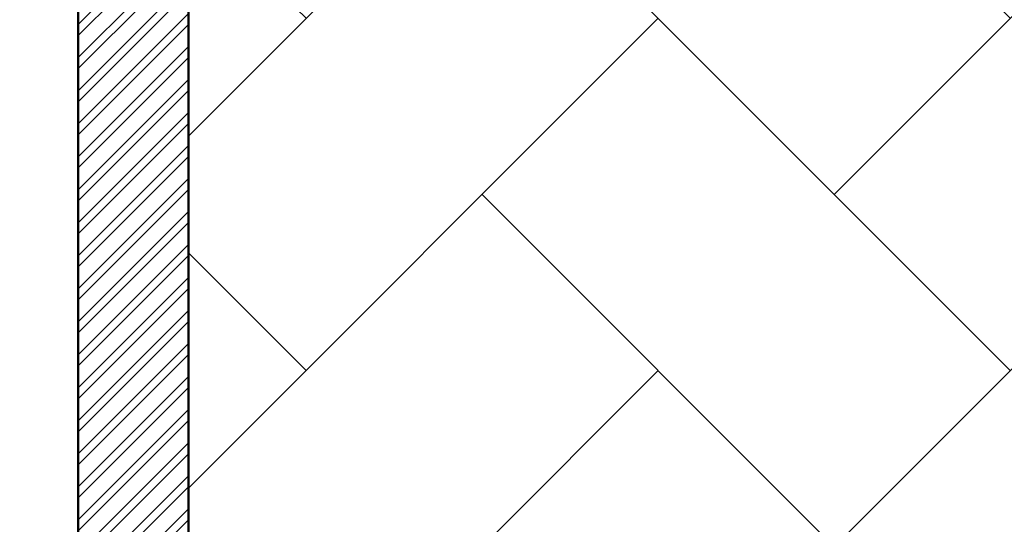
# Model space of a CAD drawing. Units: inches. Extents: x 3590 to 5167, y 65 to 1917.
# Tile 63 of 100: x 4919 to 5000, y 1640 to 1681. Entities that reach past the tile are written whole.
import ezdxf

# ---------------------------------------------------------------- set-up
doc = ezdxf.new("R2010")
doc.units = ezdxf.units.IN
for name, color, linetype, lineweight in [('A-FLOR-PATT', 8, 'Continuous', 13), ('A-WALL', 7, 'Continuous', 50), ('A-WALL-PATT', 251, 'Continuous', 13)]:
    doc.layers.add(name, color=color, linetype=linetype, lineweight=lineweight)

msp = doc.modelspace()

# ---------------------------------------------------------------- hatches: boundary and pattern name
at = {"layer": 'A-FLOR-PATT', "transparency": 33554687}
h = msp.add_hatch(dxfattribs=at)
h.set_pattern_fill('AR-HBONE', color=256, scale=0.2)
h.set_pattern_definition([(45, (-588.972, 0), (0, 28.73682), [60.96, -20.32]), (135, (-574.604, 14.368), (3e-15, 28.73682), [60.96, -20.32])])
h.paths.add_polyline_path([(5071.274, 1796.999), (4933.274, 1796.999), (4933.274, 1753.999), (4962.774, 1753.999, -0.414214), (4928.774, 1719.999), (4933.274, 1718.999), (4933.274, 1334.999), (5071.274, 1334.999)])
h.paths.add_polyline_path([(4951.78, 1521.077), (4951.715, 1521.04), (4951.563, 1520.895)], flags=16)
h.paths.add_polyline_path([(4952.267, 1521.376), (4952.198, 1521.371), (4952.198, 1521.356)], flags=0)
h.paths.add_polyline_path([(4967.051, 1529.728), (4965.231, 1528.694), (4963.411, 1527.714), (4961.756, 1526.851), (4963.589, 1527.449), (4964.036, 1527.478), (4962.975, 1527.249), (4961.76, 1526.852), (4959.792, 1525.834), (4958.005, 1524.895), (4956.24, 1523.93), (4954.504, 1522.919), (4954.129, 1522.682), (4953.361, 1521.997), (4953.366, 1521.998), (4953.605, 1522.064), (4955.106, 1522.761), (4956.921, 1523.434), (4958.678, 1523.915), (4960.358, 1524.2), (4961.945, 1524.286), (4964.171, 1524.108), (4965.958, 1523.309), (4963.863, 1522.976), (4965.187, 1522.499), (4963.366, 1522.497), (4961.545, 1522.487), (4959.764, 1522.461), (4958.304, 1522.419), (4957.974, 1522.388), (4956.307, 1522.232), (4954.718, 1522.071), (4953.251, 1521.899), (4953.525, 1521.623), (4954.331, 1521.379), (4956.243, 1521.23), (4958.039, 1520.93), (4959.684, 1520.483), (4961.16, 1519.896), (4963.107, 1518.8), (4964.393, 1517.325), (4962.973, 1517.726), (4964.558, 1516.661), (4965.407, 1515.708), (4963.507, 1516.322), (4961.68, 1517.005), (4959.935, 1517.745), (4958.282, 1518.528), (4956.732, 1519.343), (4955.295, 1520.175), (4954.672, 1520.572), (4954.513, 1520.627), (4955.658, 1519.318), (4956.703, 1517.982), (4957.644, 1516.647), (4958.485, 1515.334), (4959.55, 1513.524), (4960.438, 1511.769), (4958.841, 1513.62), (4957.452, 1515.325), (4955.819, 1517.459), (4956.665, 1515.448), (4957.111, 1513.923), (4957.447, 1511.714), (4957.076, 1509.793), (4956.538, 1511.11), (4955.992, 1512.569), (4955.444, 1514.125), (4954.898, 1515.735), (4954.357, 1517.356), (4953.824, 1518.943), (4953.305, 1520.452), (4953.065, 1521.116), (4952.971, 1521.146), (4952.949, 1521.086), (4952.73, 1520.199), (4953.37, 1518.024), (4953.757, 1516.373), (4954.051, 1514.765), (4954.264, 1513.221), (4954.471, 1511.131), (4954.497, 1510.402), (4954.409, 1511.76), (4954.264, 1513.221), (4954.051, 1514.765), (4953.757, 1516.373), (4953.37, 1518.024), (4952.877, 1519.698), (4952.716, 1520.141), (4952.533, 1519.059), (4952.374, 1517.789), (4952.219, 1516.312), (4952.046, 1514.6), (4951.833, 1512.626), (4951.557, 1510.363), (4951.203, 1512.168), (4950.852, 1514.339), (4950.985, 1516.376), (4951.66, 1518.286), (4952.593, 1520.481), (4952.357, 1521.13), (4951.855, 1520.328), (4950.839, 1518.908), (4949.777, 1517.587), (4948.916, 1516.617), (4948.111, 1515.256), (4947.089, 1513.554), (4945.889, 1511.615), (4946.326, 1513.402), (4946.562, 1514.249), (4945.528, 1513.327), (4944.581, 1512.531), (4946.018, 1514.508), (4947.204, 1516.048), (4947.893, 1517.313), (4949.307, 1518.764), (4950.414, 1519.767), (4950.451, 1519.806), (4952.267, 1521.376), (4951.645, 1521.493), (4950.404, 1521.18), (4948.044, 1520.359), (4946.119, 1519.452), (4944.572, 1518.475), (4943.35, 1517.443), (4941.997, 1515.92), (4941.661, 1515.275), (4942.813, 1516.99), (4944.572, 1518.475), (4946.119, 1519.452), (4948.044, 1520.359), (4950.404, 1521.18), (4951.645, 1521.493), (4949.647, 1521.868), (4948.6, 1521.756), (4947.126, 1521.57), (4945.42, 1521.348), (4943.45, 1521.105), (4941.183, 1520.856), (4942.86, 1521.613), (4943.873, 1522.03), (4942.952, 1521.909), (4941.41, 1521.485), (4939.543, 1520.67), (4938.968, 1520.226), (4940.733, 1521.299), (4942.952, 1521.909), (4943.702, 1522.008), (4945.894, 1522.7), (4947.565, 1522.714), (4948.921, 1522.566), (4951.131, 1522.183), (4950.971, 1522.297), (4948.129, 1523.006), (4946.035, 1523.707), (4944.232, 1524.521), (4942.707, 1525.461), (4941.444, 1526.537), (4940.43, 1527.761), (4939.649, 1529.143), (4941.421, 1528.122), (4943.147, 1527.132), (4944.841, 1526.175), (4946.514, 1525.25), (4948.179, 1524.359), (4948.365, 1524.263), (4946.475, 1526.045), (4945.181, 1527.54), (4944.19, 1529.033), (4943.496, 1530.54), (4943.278, 1531.36), (4942.498, 1531.919), (4943.114, 1531.762), (4942.959, 1533.659), (4944.14, 1531.989), (4944.612, 1531.323), (4946.202, 1530.463), (4947.486, 1529.509), (4948.79, 1528.226), (4950.368, 1526.237), (4949.485, 1528.155), (4948.851, 1530.123), (4948.491, 1532.041), (4948.381, 1533.918), (4948.501, 1535.76), (4948.827, 1537.573), (4949.418, 1535.565), (4949.957, 1533.569), (4950.464, 1531.586), (4950.961, 1529.617), (4951.391, 1527.954), (4951.724, 1530.687), (4952.201, 1532.58), (4952.889, 1534.33), (4953.77, 1535.951), (4954.827, 1537.46), (4954.521, 1535.39), (4954.273, 1533.937), (4955.58, 1535.663), (4956.748, 1536.739), (4956.159, 1534.78), (4955.589, 1532.873), (4955.043, 1531.006), (4954.525, 1529.166), (4954.038, 1527.341), (4953.638, 1525.733), (4953.611, 1525.586), (4953.398, 1524.166), (4953.382, 1524.009), (4954.07, 1525.476), (4954.912, 1527.022), (4956.136, 1528.894), (4957.847, 1530.577), (4959.376, 1531.54), (4958.256, 1530.104), (4957.143, 1528.663), (4956.066, 1527.243), (4955.056, 1525.871), (4954.141, 1524.571), (4953.352, 1523.372), (4953.311, 1523.303), (4953.273, 1522.925), (4953.261, 1522.382), (4954.103, 1523.373), (4954.63, 1524.284), (4955.961, 1526.358), (4957.23, 1528.13), (4958.421, 1529.609), (4960.037, 1531.368), (4961.374, 1532.375), (4962.101, 1532.77), (4961.07, 1531.061), (4959.987, 1529.438), (4958.869, 1527.908), (4958.15, 1527.007), (4959.803, 1528.003), (4961.589, 1528.793), (4963.391, 1529.328), (4965.211, 1529.632)], flags=16)
h.paths.add_polyline_path([(4962.944, 1523.182), (4961.107, 1523.422), (4960.392, 1523.362), (4962.35, 1523.331)], flags=0)
h.paths.add_polyline_path([(5049.541, 1584.551), (5049.476, 1584.515), (5049.325, 1584.37)], flags=16)
h.paths.add_polyline_path([(5050.028, 1584.851), (5049.959, 1584.845), (5049.959, 1584.83)], flags=0)
h.paths.add_polyline_path([(5042.333, 1581.949), (5043.88, 1582.926), (5045.806, 1583.833), (5048.165, 1584.654), (5049.406, 1584.967), (5047.408, 1585.342), (5046.361, 1585.231), (5044.888, 1585.044), (5043.181, 1584.822), (5041.211, 1584.579), (5038.944, 1584.33), (5040.622, 1585.087), (5041.634, 1585.504), (5040.713, 1585.383), (5039.171, 1584.959), (5037.304, 1584.144), (5036.729, 1583.7), (5038.494, 1584.773), (5040.713, 1585.383), (5041.463, 1585.482), (5043.655, 1586.174), (5045.326, 1586.188), (5046.682, 1586.04), (5048.893, 1585.657), (5048.732, 1585.771), (5045.891, 1586.48), (5043.796, 1587.181), (5041.994, 1587.996), (5040.468, 1588.935), (5039.205, 1590.011), (5038.191, 1591.235), (5037.41, 1592.617), (5039.182, 1591.596), (5040.909, 1590.607), (5042.602, 1589.649), (5044.275, 1588.724), (5045.94, 1587.833), (5046.126, 1587.738), (5044.237, 1589.519), (5042.942, 1591.015), (5041.952, 1592.508), (5041.257, 1594.014), (5041.039, 1594.834), (5040.26, 1595.393), (5040.875, 1595.237), (5040.721, 1597.133), (5041.901, 1595.463), (5042.373, 1594.798), (5043.963, 1593.938), (5045.247, 1592.983), (5046.552, 1591.701), (5048.129, 1589.712), (5047.247, 1591.63), (5046.613, 1593.597), (5046.252, 1595.515), (5046.142, 1597.392), (5046.262, 1599.234), (5046.588, 1601.047), (5047.179, 1599.039), (5047.718, 1597.043), (5048.225, 1595.06), (5048.722, 1593.091), (5049.152, 1591.429), (5049.485, 1594.161), (5049.962, 1596.054), (5050.65, 1597.804), (5051.532, 1599.425), (5052.589, 1600.934), (5052.283, 1598.864), (5052.034, 1597.411), (5053.341, 1599.137), (5054.509, 1600.213), (5053.92, 1598.254), (5053.35, 1596.348), (5052.805, 1594.48), (5052.286, 1592.64), (5051.799, 1590.815), (5051.4, 1589.207), (5051.373, 1589.06), (5051.159, 1587.64), (5051.143, 1587.483), (5051.831, 1588.95), (5052.673, 1590.496), (5053.898, 1592.368), (5055.608, 1594.051), (5057.137, 1595.014), (5056.017, 1593.578), (5054.904, 1592.137), (5053.828, 1590.717), (5052.817, 1589.345), (5051.902, 1588.046), (5051.113, 1586.846), (5051.072, 1586.777), (5051.034, 1586.399), (5051.022, 1585.856), (5051.864, 1586.847), (5052.391, 1587.758), (5053.723, 1589.832), (5054.991, 1591.604), (5056.182, 1593.083), (5057.798, 1594.842), (5059.135, 1595.849), (5059.863, 1596.244), (5058.831, 1594.535), (5057.749, 1592.912), (5056.63, 1591.382), (5055.912, 1590.482), (5057.564, 1591.477), (5059.35, 1592.267), (5061.152, 1592.802), (5062.972, 1593.106), (5064.812, 1593.203), (5062.992, 1592.169), (5061.172, 1591.188), (5059.518, 1590.325), (5061.35, 1590.924), (5061.797, 1590.952), (5060.737, 1590.723), (5059.521, 1590.326), (5057.553, 1589.308), (5055.766, 1588.369), (5054.002, 1587.404), (5052.265, 1586.393), (5051.891, 1586.156), (5051.122, 1585.471), (5051.127, 1585.472), (5051.366, 1585.538), (5052.867, 1586.235), (5054.682, 1586.908), (5056.439, 1587.389), (5058.12, 1587.675), (5059.706, 1587.76), (5061.933, 1587.583), (5063.719, 1586.783), (5061.624, 1586.45), (5062.949, 1585.973), (5061.127, 1585.971), (5059.307, 1585.961), (5057.525, 1585.935), (5056.065, 1585.893), (5055.735, 1585.862), (5054.068, 1585.707), (5052.479, 1585.546), (5051.012, 1585.373), (5051.286, 1585.097), (5052.092, 1584.853), (5054.004, 1584.704), (5055.8, 1584.404), (5057.446, 1583.958), (5058.921, 1583.37), (5060.868, 1582.274), (5062.154, 1580.799), (5060.734, 1581.2), (5062.32, 1580.135), (5063.168, 1579.182), (5061.269, 1579.796), (5059.441, 1580.479), (5057.696, 1581.219), (5056.043, 1582.003), (5054.493, 1582.817), (5053.057, 1583.649), (5052.433, 1584.047), (5052.274, 1584.101), (5053.42, 1582.793), (5054.464, 1581.457), (5055.405, 1580.121), (5056.247, 1578.809), (5057.311, 1576.998), (5058.199, 1575.244), (5056.602, 1577.094), (5055.213, 1578.799), (5053.58, 1580.933), (5054.427, 1578.922), (5054.872, 1577.397), (5055.208, 1575.189), (5054.838, 1573.267), (5054.299, 1574.584), (5053.754, 1576.043), (5053.206, 1577.599), (5052.659, 1579.209), (5052.118, 1580.83), (5051.585, 1582.417), (5051.066, 1583.927), (5050.826, 1584.59), (5050.733, 1584.62), (5050.711, 1584.561), (5050.491, 1583.673), (5051.131, 1581.498), (5051.518, 1579.847), (5051.813, 1578.24), (5052.026, 1576.695), (5052.233, 1574.605), (5052.258, 1573.876), (5052.17, 1575.234), (5052.026, 1576.695), (5051.813, 1578.24), (5051.518, 1579.847), (5051.131, 1581.498), (5050.638, 1583.172), (5050.477, 1583.615), (5050.294, 1582.533), (5050.136, 1581.263), (5049.981, 1579.786), (5049.807, 1578.074), (5049.594, 1576.1), (5049.318, 1573.837), (5048.965, 1575.642), (5048.613, 1577.813), (5048.747, 1579.85), (5049.421, 1581.76), (5050.354, 1583.955), (5050.118, 1584.604), (5049.616, 1583.802), (5048.6, 1582.382), (5047.538, 1581.061), (5046.677, 1580.091), (5045.872, 1578.73), (5044.85, 1577.028), (5043.651, 1575.089), (5044.087, 1576.877), (5044.324, 1577.723), (5043.289, 1576.801), (5042.342, 1576.005), (5043.779, 1577.982), (5044.966, 1579.522), (5045.655, 1580.787), (5047.068, 1582.239), (5048.175, 1583.241), (5048.213, 1583.28), (5050.028, 1584.851), (5049.406, 1584.967), (5048.165, 1584.654), (5045.806, 1583.833), (5043.88, 1582.926), (5042.333, 1581.949), (5041.111, 1580.917), (5039.758, 1579.394), (5039.423, 1578.749), (5040.575, 1580.464)], flags=16)
h.paths.add_polyline_path([(4954.799, 1533.12), (4954.262, 1532.079), (4953.831, 1530.935), (4953.505, 1529.636), (4953.283, 1528.133), (4953.167, 1526.376), (4953.156, 1524.315), (4953.277, 1521.236), (4952.802, 1521.842), (4951.557, 1521.998), (4950.976, 1521.961), (4952.661, 1521.941), (4952.802, 1521.842), (4953.152, 1523.593), (4953.167, 1526.376), (4953.283, 1528.133), (4953.609, 1530.346), (4954.456, 1532.592)], flags=0)
h.paths.add_polyline_path([(5050.563, 1585.316), (5049.318, 1585.472), (5048.737, 1585.435), (5050.422, 1585.415), (5050.563, 1585.316), (5050.914, 1587.067), (5050.928, 1589.851), (5051.045, 1591.607), (5051.371, 1593.82), (5052.217, 1596.066), (5052.56, 1596.594), (5052.024, 1595.554), (5051.592, 1594.409), (5051.266, 1593.11), (5051.045, 1591.607), (5050.928, 1589.851), (5050.918, 1587.789), (5051.038, 1584.71)], flags=0)
h.paths.add_polyline_path([(5058.153, 1586.836), (5060.111, 1586.805), (5060.705, 1586.656), (5058.868, 1586.896)], flags=0)
h.paths.add_polyline_path([(5049.541, 1430.936), (5049.476, 1430.9), (5049.325, 1430.755)], flags=16)
h.paths.add_polyline_path([(5050.028, 1431.236), (5049.959, 1431.231), (5049.959, 1431.215)], flags=0)
h.paths.add_polyline_path([(5046.588, 1447.432), (5047.179, 1445.425), (5047.718, 1443.429), (5048.225, 1441.446), (5048.722, 1439.476), (5049.152, 1437.814), (5049.485, 1440.546), (5049.962, 1442.439), (5050.65, 1444.189), (5051.532, 1445.811), (5052.589, 1447.319), (5052.283, 1445.249), (5052.034, 1443.796), (5053.341, 1445.522), (5054.509, 1446.598), (5053.92, 1444.64), (5053.35, 1442.733), (5052.805, 1440.865), (5052.286, 1439.025), (5051.799, 1437.201), (5051.4, 1435.592), (5051.373, 1435.445), (5051.159, 1434.025), (5051.143, 1433.868), (5051.831, 1435.335), (5052.673, 1436.881), (5053.898, 1438.753), (5055.608, 1440.436), (5057.137, 1441.4), (5056.017, 1439.963), (5054.904, 1438.522), (5053.828, 1437.102), (5052.817, 1435.73), (5051.902, 1434.431), (5051.113, 1433.231), (5051.072, 1433.162), (5051.034, 1432.784), (5051.022, 1432.242), (5051.864, 1433.232), (5052.391, 1434.143), (5053.723, 1436.217), (5054.991, 1437.989), (5056.182, 1439.468), (5057.798, 1441.227), (5059.135, 1442.235), (5059.863, 1442.629), (5058.831, 1440.921), (5057.749, 1439.298), (5056.63, 1437.767), (5055.912, 1436.867), (5057.564, 1437.863), (5059.35, 1438.652), (5061.152, 1439.187), (5062.972, 1439.491), (5064.812, 1439.588), (5062.992, 1438.554), (5061.172, 1437.573), (5059.518, 1436.71), (5061.35, 1437.309), (5061.797, 1437.337), (5060.737, 1437.108), (5059.521, 1436.711), (5057.553, 1435.693), (5055.766, 1434.754), (5054.002, 1433.789), (5052.265, 1432.778), (5051.891, 1432.541), (5051.122, 1431.856), (5051.127, 1431.857), (5051.366, 1431.923), (5052.867, 1432.62), (5054.682, 1433.293), (5056.439, 1433.775), (5058.12, 1434.06), (5059.706, 1434.145), (5061.933, 1433.968), (5063.719, 1433.168), (5061.624, 1432.835), (5062.949, 1432.358), (5061.127, 1432.357), (5059.307, 1432.346), (5057.525, 1432.32), (5056.065, 1432.278), (5055.735, 1432.248), (5054.068, 1432.092), (5052.479, 1431.931), (5051.012, 1431.759), (5051.286, 1431.482), (5052.092, 1431.238), (5054.004, 1431.089), (5055.8, 1430.789), (5057.446, 1430.343), (5058.921, 1429.755), (5060.868, 1428.66), (5062.154, 1427.185), (5060.734, 1427.585), (5062.32, 1426.52), (5063.168, 1425.567), (5061.269, 1426.181), (5059.441, 1426.865), (5057.696, 1427.604), (5056.043, 1428.388), (5054.493, 1429.202), (5053.057, 1430.034), (5052.433, 1430.432), (5052.274, 1430.487), (5053.42, 1429.178), (5054.464, 1427.842), (5055.405, 1426.506), (5056.247, 1425.194), (5057.311, 1423.383), (5058.199, 1421.629), (5056.602, 1423.479), (5055.213, 1425.184), (5053.58, 1427.318), (5054.427, 1425.307), (5054.872, 1423.782), (5055.208, 1421.574), (5054.838, 1419.652), (5054.299, 1420.97), (5053.754, 1422.428), (5053.206, 1423.984), (5052.659, 1425.595), (5052.118, 1427.215), (5051.585, 1428.802), (5051.066, 1430.312), (5050.826, 1430.975), (5050.733, 1431.005), (5050.711, 1430.946), (5050.491, 1430.058), (5051.131, 1427.883), (5051.518, 1426.232), (5051.813, 1424.625), (5052.026, 1423.081), (5052.233, 1420.991), (5052.258, 1420.261), (5052.17, 1421.619), (5052.026, 1423.081), (5051.813, 1424.625), (5051.518, 1426.232), (5051.131, 1427.883), (5050.638, 1429.558), (5050.477, 1430.001), (5050.294, 1428.918), (5050.136, 1427.648), (5049.981, 1426.171), (5049.807, 1424.459), (5049.594, 1422.485), (5049.318, 1420.222), (5048.965, 1422.028), (5048.613, 1424.199), (5048.747, 1426.235), (5049.421, 1428.146), (5050.354, 1430.34), (5050.118, 1430.989), (5049.616, 1430.187), (5048.6, 1428.768), (5047.538, 1427.446), (5046.677, 1426.477), (5045.872, 1425.116), (5044.85, 1423.413), (5043.651, 1421.474), (5044.087, 1423.262), (5044.324, 1424.109), (5043.289, 1423.186), (5042.342, 1422.391), (5043.779, 1424.368), (5044.966, 1425.907), (5045.655, 1427.173), (5047.068, 1428.624), (5048.175, 1429.627), (5048.213, 1429.666), (5050.028, 1431.236), (5049.406, 1431.353), (5048.165, 1431.039), (5045.806, 1430.218), (5043.88, 1429.311), (5042.333, 1428.334), (5041.111, 1427.302), (5039.758, 1425.779), (5039.423, 1425.134), (5040.575, 1426.849), (5042.333, 1428.334), (5043.88, 1429.311), (5045.806, 1430.218), (5048.165, 1431.039), (5049.406, 1431.353), (5047.408, 1431.727), (5046.361, 1431.616), (5044.888, 1431.429), (5043.181, 1431.207), (5041.211, 1430.964), (5038.944, 1430.715), (5040.622, 1431.472), (5041.634, 1431.89), (5040.713, 1431.769), (5039.171, 1431.345), (5037.304, 1430.53), (5036.729, 1430.085), (5038.494, 1431.158), (5040.713, 1431.769), (5041.463, 1431.867), (5043.655, 1432.559), (5045.326, 1432.573), (5046.682, 1432.425), (5048.893, 1432.042), (5048.732, 1432.156), (5045.891, 1432.865), (5043.796, 1433.566), (5041.994, 1434.381), (5040.468, 1435.321), (5039.205, 1436.396), (5038.191, 1437.62), (5037.41, 1439.002), (5039.182, 1437.982), (5040.909, 1436.992), (5042.602, 1436.034), (5044.275, 1435.109), (5045.94, 1434.218), (5046.126, 1434.123), (5044.237, 1435.904), (5042.942, 1437.4), (5041.952, 1438.893), (5041.257, 1440.399), (5041.039, 1441.219), (5040.26, 1441.778), (5040.875, 1441.622), (5040.721, 1443.518), (5041.901, 1441.848), (5042.373, 1441.183), (5043.963, 1440.323), (5045.247, 1439.369), (5046.552, 1438.086), (5048.129, 1436.097), (5047.247, 1438.015), (5046.613, 1439.982), (5046.252, 1441.901), (5046.142, 1443.778), (5046.262, 1445.619)], flags=16)
h.paths.add_polyline_path([(5052.382, 1444.255), (5051.623, 1442.78), (5052.024, 1441.939), (5052.56, 1442.98)], flags=0)
h.paths.add_polyline_path([(5050.563, 1431.701), (5049.318, 1431.857), (5048.737, 1431.821), (5050.422, 1431.8)], flags=0)
h.paths.add_polyline_path([(5058.153, 1433.221), (5060.111, 1433.19), (5060.705, 1433.041), (5058.868, 1433.281)], flags=0)
h.paths.add_polyline_path([(5049.541, 1352.285), (5049.476, 1352.249), (5049.325, 1352.104)], flags=16)
h.paths.add_polyline_path([(5050.028, 1352.585), (5049.959, 1352.58), (5049.959, 1352.564)], flags=0)
h.paths.add_polyline_path([(5046.588, 1368.781), (5047.179, 1366.774), (5047.718, 1364.778), (5048.225, 1362.795), (5048.722, 1360.825), (5049.152, 1359.163), (5049.485, 1361.896), (5049.962, 1363.789), (5050.65, 1365.538), (5051.532, 1367.16), (5052.589, 1368.669), (5052.283, 1366.598), (5052.034, 1365.145), (5053.341, 1366.871), (5054.509, 1367.947), (5053.92, 1365.989), (5053.35, 1364.082), (5052.805, 1362.214), (5052.286, 1360.374), (5051.799, 1358.55), (5051.4, 1356.942), (5051.373, 1356.794), (5051.159, 1355.374), (5051.143, 1355.218), (5051.831, 1356.684), (5052.673, 1358.23), (5053.898, 1360.102), (5055.608, 1361.786), (5057.137, 1362.749), (5056.017, 1361.313), (5054.904, 1359.872), (5053.828, 1358.452), (5052.817, 1357.079), (5051.902, 1355.78), (5051.113, 1354.581), (5051.072, 1354.512), (5051.034, 1354.133), (5051.022, 1353.591), (5051.864, 1354.581), (5052.391, 1355.492), (5053.723, 1357.566), (5054.991, 1359.338), (5056.182, 1360.817), (5057.798, 1362.577), (5059.135, 1363.584), (5059.863, 1363.979), (5058.831, 1362.27), (5057.749, 1360.647), (5056.63, 1359.117), (5055.912, 1358.216), (5057.564, 1359.212), (5059.35, 1360.001), (5061.152, 1360.536), (5062.972, 1360.841), (5064.812, 1360.937), (5062.992, 1359.903), (5061.172, 1358.923), (5059.518, 1358.059), (5061.35, 1358.658), (5061.797, 1358.687), (5060.737, 1358.458), (5059.521, 1358.061), (5057.553, 1357.043), (5055.766, 1356.103), (5054.002, 1355.138), (5052.265, 1354.127), (5051.891, 1353.89), (5051.122, 1353.206), (5051.127, 1353.206), (5051.366, 1353.272), (5052.867, 1353.969), (5054.682, 1354.643), (5056.439, 1355.124), (5058.12, 1355.409), (5059.706, 1355.495), (5061.933, 1355.317), (5063.719, 1354.518), (5061.624, 1354.184), (5062.949, 1353.708), (5061.127, 1353.706), (5059.307, 1353.695), (5057.525, 1353.669), (5056.065, 1353.627), (5055.735, 1353.597), (5054.068, 1353.441), (5052.479, 1353.28), (5051.012, 1353.108), (5051.286, 1352.831), (5052.092, 1352.587), (5054.004, 1352.439), (5055.8, 1352.138), (5057.446, 1351.692), (5058.921, 1351.104), (5060.868, 1350.009), (5062.154, 1348.534), (5060.734, 1348.935), (5062.32, 1347.869), (5063.168, 1346.916), (5061.269, 1347.53), (5059.441, 1348.214), (5057.696, 1348.954), (5056.043, 1349.737), (5054.493, 1350.551), (5053.057, 1351.383), (5052.433, 1351.781), (5052.274, 1351.836), (5053.42, 1350.527), (5054.464, 1349.191), (5055.405, 1347.855), (5056.247, 1346.543), (5057.311, 1344.733), (5058.199, 1342.978), (5056.602, 1344.828), (5055.213, 1346.534), (5053.58, 1348.667), (5054.427, 1346.656), (5054.872, 1345.132), (5055.208, 1342.923), (5054.838, 1341.002), (5054.299, 1342.319), (5053.754, 1343.778), (5053.206, 1345.334), (5052.659, 1346.944), (5052.118, 1348.564), (5051.585, 1350.151), (5051.066, 1351.661), (5050.826, 1352.324), (5050.733, 1352.355), (5050.711, 1352.295), (5050.491, 1351.408), (5051.131, 1349.232), (5051.518, 1347.581), (5051.813, 1345.974), (5052.026, 1344.43), (5052.233, 1342.34), (5052.258, 1341.61), (5052.17, 1342.969), (5052.026, 1344.43), (5051.813, 1345.974), (5051.518, 1347.581), (5051.131, 1349.232), (5050.638, 1350.907), (5050.477, 1351.35), (5050.294, 1350.267), (5050.136, 1348.997), (5049.981, 1347.52), (5049.807, 1345.809), (5049.594, 1343.835), (5049.318, 1341.571), (5048.965, 1343.377), (5048.613, 1345.548), (5048.747, 1347.585), (5049.421, 1349.495), (5050.354, 1351.689), (5050.118, 1352.339), (5049.616, 1351.536), (5048.6, 1350.117), (5047.538, 1348.795), (5046.677, 1347.826), (5045.872, 1346.465), (5044.85, 1344.763), (5043.651, 1342.824), (5044.087, 1344.611), (5044.324, 1345.458), (5043.289, 1344.535), (5042.342, 1343.74), (5043.779, 1345.717), (5044.966, 1347.256), (5045.655, 1348.522), (5047.068, 1349.973), (5048.175, 1350.976), (5048.213, 1351.015), (5050.028, 1352.585), (5049.406, 1352.702), (5048.165, 1352.388), (5045.806, 1351.567), (5043.88, 1350.661), (5042.333, 1349.683), (5041.111, 1348.651), (5039.758, 1347.128), (5039.423, 1346.483), (5040.575, 1348.198), (5042.333, 1349.683), (5043.88, 1350.661), (5045.806, 1351.567), (5048.165, 1352.388), (5049.406, 1352.702), (5047.408, 1353.076), (5046.361, 1352.965), (5044.888, 1352.779), (5043.181, 1352.556), (5041.211, 1352.313), (5038.944, 1352.065), (5040.622, 1352.821), (5041.634, 1353.239), (5040.713, 1353.118), (5039.171, 1352.694), (5037.304, 1351.879), (5036.729, 1351.434), (5038.494, 1352.508), (5040.713, 1353.118), (5041.463, 1353.216), (5043.655, 1353.909), (5045.326, 1353.923), (5046.682, 1353.774), (5048.893, 1353.391), (5048.732, 1353.506), (5045.891, 1354.214), (5043.796, 1354.915), (5041.994, 1355.73), (5040.468, 1356.67), (5039.205, 1357.746), (5038.191, 1358.969), (5037.41, 1360.352), (5039.182, 1359.331), (5040.909, 1358.341), (5042.602, 1357.383), (5044.275, 1356.458), (5045.94, 1355.567), (5046.126, 1355.472), (5044.237, 1357.253), (5042.942, 1358.749), (5041.952, 1360.242), (5041.257, 1361.748), (5041.039, 1362.568), (5040.26, 1363.128), (5040.875, 1362.971), (5040.721, 1364.867), (5041.901, 1363.197), (5042.373, 1362.532), (5043.963, 1361.672), (5045.247, 1360.718), (5046.552, 1359.435), (5048.129, 1357.446), (5047.247, 1359.364), (5046.613, 1361.331), (5046.252, 1363.25), (5046.142, 1365.127), (5046.262, 1366.969)], flags=16)
h.paths.add_polyline_path([(5052.382, 1365.604), (5051.623, 1364.129), (5052.024, 1363.288), (5052.56, 1364.329)], flags=0)
h.paths.add_polyline_path([(4951.78, 1698.041), (4951.715, 1698.005), (4951.563, 1697.859)], flags=16)
h.paths.add_polyline_path([(4952.267, 1698.341), (4952.198, 1698.335), (4952.198, 1698.32)], flags=0)
h.paths.add_polyline_path([(4957.076, 1686.757), (4956.538, 1688.074), (4955.992, 1689.533), (4955.444, 1691.089), (4954.898, 1692.699), (4954.357, 1694.32), (4953.824, 1695.907), (4953.305, 1697.417), (4953.065, 1698.08), (4952.971, 1698.11), (4952.949, 1698.051), (4952.73, 1697.163), (4953.37, 1694.988), (4953.757, 1693.337), (4954.051, 1691.729), (4954.264, 1690.185), (4954.471, 1688.095), (4954.497, 1687.366), (4954.409, 1688.724), (4954.264, 1690.185), (4954.051, 1691.729), (4953.757, 1693.337), (4953.37, 1694.988), (4952.877, 1696.662), (4952.716, 1697.105), (4952.533, 1696.023), (4952.374, 1694.753), (4952.219, 1693.276), (4952.046, 1691.564), (4951.833, 1689.59), (4951.557, 1687.327), (4951.203, 1689.132), (4950.852, 1691.303), (4950.985, 1693.34), (4951.66, 1695.25), (4952.593, 1697.445), (4952.357, 1698.094), (4951.855, 1697.292), (4950.839, 1695.872), (4949.777, 1694.551), (4948.916, 1693.581), (4948.111, 1692.22), (4947.089, 1690.518), (4945.889, 1688.579), (4946.326, 1690.366), (4946.562, 1691.213), (4945.528, 1690.291), (4944.581, 1689.495), (4946.018, 1691.472), (4947.204, 1693.012), (4947.893, 1694.277), (4949.307, 1695.729), (4950.414, 1696.731), (4950.451, 1696.77), (4952.267, 1698.341), (4951.645, 1698.457), (4950.404, 1698.144), (4948.044, 1697.323), (4946.119, 1696.416), (4944.572, 1695.439), (4943.35, 1694.407), (4941.997, 1692.884), (4941.661, 1692.239), (4942.813, 1693.954), (4944.572, 1695.439), (4946.119, 1696.416), (4948.044, 1697.323), (4950.404, 1698.144), (4951.645, 1698.457), (4949.647, 1698.832), (4948.6, 1698.72), (4947.126, 1698.534), (4945.42, 1698.312), (4943.45, 1698.069), (4941.183, 1697.82), (4942.86, 1698.577), (4943.873, 1698.994), (4942.952, 1698.873), (4941.41, 1698.449), (4939.543, 1697.634), (4938.968, 1697.19), (4940.733, 1698.263), (4942.952, 1698.873), (4943.702, 1698.972), (4945.894, 1699.664), (4947.565, 1699.678), (4948.921, 1699.53), (4951.131, 1699.147), (4950.971, 1699.261), (4948.129, 1699.97), (4946.035, 1700.671), (4944.232, 1701.486), (4942.707, 1702.425), (4941.444, 1703.501), (4940.43, 1704.725), (4939.649, 1706.107), (4941.421, 1705.086), (4943.147, 1704.097), (4944.841, 1703.139), (4946.514, 1702.214), (4948.179, 1701.323), (4948.365, 1701.227), (4946.475, 1703.009), (4945.181, 1704.505), (4944.19, 1705.997), (4943.496, 1707.504), (4943.278, 1708.324), (4942.498, 1708.883), (4943.114, 1708.727), (4942.959, 1710.623), (4944.14, 1708.953), (4944.612, 1708.287), (4946.202, 1707.428), (4947.486, 1706.473), (4948.79, 1705.191), (4950.368, 1703.202), (4949.485, 1705.12), (4948.851, 1707.087), (4948.491, 1709.005), (4948.381, 1710.882), (4948.501, 1712.724), (4948.827, 1714.537), (4949.418, 1712.529), (4949.957, 1710.533), (4950.464, 1708.55), (4950.961, 1706.581), (4951.391, 1704.919), (4951.724, 1707.651), (4952.201, 1709.544), (4952.889, 1711.294), (4953.77, 1712.915), (4954.827, 1714.424), (4954.521, 1712.354), (4954.273, 1710.901), (4955.58, 1712.627), (4956.748, 1713.703), (4956.159, 1711.744), (4955.589, 1709.837), (4955.043, 1707.97), (4954.525, 1706.13), (4954.038, 1704.305), (4953.638, 1702.697), (4953.611, 1702.55), (4953.398, 1701.13), (4953.382, 1700.973), (4954.07, 1702.44), (4954.912, 1703.986), (4956.136, 1705.858), (4957.847, 1707.541), (4959.376, 1708.504), (4958.256, 1707.068), (4957.143, 1705.627), (4956.066, 1704.207), (4955.056, 1702.835), (4954.141, 1701.536), (4953.352, 1700.336), (4953.311, 1700.267), (4953.273, 1699.889), (4953.261, 1699.346), (4954.103, 1700.337), (4954.63, 1701.248), (4955.961, 1703.322), (4957.23, 1705.094), (4958.421, 1706.573), (4960.037, 1708.332), (4961.374, 1709.339), (4962.101, 1709.734), (4961.07, 1708.025), (4959.987, 1706.402), (4958.869, 1704.872), (4958.15, 1703.972), (4959.803, 1704.967), (4961.589, 1705.757), (4963.391, 1706.292), (4965.211, 1706.596), (4967.051, 1706.692), (4965.231, 1705.659), (4963.411, 1704.678), (4961.756, 1703.815), (4963.589, 1704.413), (4964.036, 1704.442), (4962.975, 1704.213), (4961.76, 1703.816), (4959.792, 1702.798), (4958.005, 1701.859), (4956.24, 1700.894), (4954.504, 1699.883), (4954.129, 1699.646), (4953.361, 1698.961), (4953.366, 1698.962), (4953.605, 1699.028), (4955.106, 1699.725), (4956.921, 1700.398), (4958.678, 1700.879), (4960.358, 1701.164), (4961.945, 1701.25), (4964.171, 1701.073), (4965.958, 1700.273), (4963.863, 1699.94), (4965.187, 1699.463), (4963.366, 1699.461), (4961.545, 1699.451), (4959.764, 1699.425), (4958.304, 1699.383), (4957.974, 1699.352), (4956.307, 1699.197), (4954.718, 1699.036), (4953.251, 1698.863), (4953.525, 1698.587), (4954.331, 1698.343), (4956.243, 1698.194), (4958.039, 1697.894), (4959.684, 1697.447), (4961.16, 1696.86), (4963.107, 1695.764), (4964.393, 1694.289), (4962.973, 1694.69), (4964.558, 1693.625), (4965.407, 1692.672), (4963.507, 1693.286), (4961.68, 1693.969), (4959.935, 1694.709), (4958.282, 1695.492), (4956.732, 1696.307), (4955.295, 1697.139), (4954.672, 1697.536), (4954.513, 1697.591), (4955.658, 1696.282), (4956.703, 1694.946), (4957.644, 1693.611), (4958.485, 1692.298), (4959.55, 1690.488), (4960.438, 1688.733), (4958.841, 1690.584), (4957.452, 1692.289), (4955.819, 1694.423), (4956.665, 1692.412), (4957.111, 1690.887), (4957.447, 1688.678)], flags=16)
h.paths.add_polyline_path([(5050.563, 1353.05), (5049.318, 1353.207), (5048.737, 1353.17), (5050.422, 1353.15)], flags=0)
h.paths.add_polyline_path([(4951.78, 1351.486), (4951.715, 1351.45), (4951.563, 1351.305)], flags=16)
h.paths.add_polyline_path([(4952.267, 1351.786), (4952.198, 1351.78), (4952.198, 1351.765)], flags=0)
h.paths.add_polyline_path([(4954.827, 1367.869), (4954.521, 1365.799), (4954.273, 1364.346), (4955.58, 1366.072), (4956.748, 1367.148), (4956.159, 1365.19), (4955.589, 1363.283), (4955.043, 1361.415), (4954.525, 1359.575), (4954.038, 1357.751), (4953.638, 1356.142), (4953.611, 1355.995), (4953.398, 1354.575), (4953.382, 1354.418), (4954.07, 1355.885), (4954.912, 1357.431), (4956.136, 1359.303), (4957.847, 1360.986), (4959.376, 1361.95), (4958.256, 1360.513), (4957.143, 1359.072), (4956.066, 1357.652), (4955.056, 1356.28), (4954.141, 1354.981), (4953.352, 1353.781), (4953.311, 1353.712), (4953.273, 1353.334), (4953.261, 1352.792), (4954.103, 1353.782), (4954.63, 1354.693), (4955.961, 1356.767), (4957.23, 1358.539), (4958.421, 1360.018), (4960.037, 1361.777), (4961.374, 1362.785), (4962.101, 1363.179), (4961.07, 1361.471), (4959.987, 1359.848), (4958.869, 1358.317), (4958.15, 1357.417), (4959.803, 1358.413), (4961.589, 1359.202), (4963.391, 1359.737), (4965.211, 1360.041), (4967.051, 1360.138), (4965.231, 1359.104), (4963.411, 1358.123), (4961.756, 1357.26), (4963.589, 1357.859), (4964.036, 1357.887), (4962.975, 1357.658), (4961.76, 1357.261), (4959.792, 1356.243), (4958.005, 1355.304), (4956.24, 1354.339), (4954.504, 1353.328), (4954.129, 1353.091), (4953.361, 1352.406), (4953.366, 1352.407), (4953.605, 1352.473), (4955.106, 1353.17), (4956.921, 1353.843), (4958.678, 1354.325), (4960.358, 1354.61), (4961.945, 1354.695), (4964.171, 1354.518), (4965.958, 1353.718), (4963.863, 1353.385), (4965.187, 1352.908), (4963.366, 1352.907), (4961.545, 1352.896), (4959.764, 1352.87), (4958.304, 1352.828), (4957.974, 1352.798), (4956.307, 1352.642), (4954.718, 1352.481), (4953.251, 1352.309), (4953.525, 1352.032), (4954.331, 1351.788), (4956.243, 1351.639), (4958.039, 1351.339), (4959.684, 1350.893), (4961.16, 1350.305), (4963.107, 1349.21), (4964.393, 1347.735), (4962.973, 1348.135), (4964.558, 1347.07), (4965.407, 1346.117), (4963.507, 1346.731), (4961.68, 1347.414), (4959.935, 1348.154), (4958.282, 1348.938), (4956.732, 1349.752), (4955.295, 1350.584), (4954.672, 1350.982), (4954.513, 1351.036), (4955.658, 1349.728), (4956.703, 1348.392), (4957.644, 1347.056), (4958.485, 1345.744), (4959.55, 1343.933), (4960.438, 1342.179), (4958.841, 1344.029), (4957.452, 1345.734), (4955.819, 1347.868), (4956.665, 1345.857), (4957.111, 1344.332), (4957.447, 1342.124), (4957.076, 1340.202), (4956.538, 1341.52), (4955.992, 1342.978), (4955.444, 1344.534), (4954.898, 1346.145), (4954.357, 1347.765), (4953.824, 1349.352), (4953.305, 1350.862), (4953.065, 1351.525), (4952.971, 1351.555), (4952.949, 1351.496), (4952.73, 1350.608), (4953.37, 1348.433), (4953.757, 1346.782), (4954.051, 1345.175), (4954.264, 1343.631), (4954.471, 1341.541), (4954.497, 1340.811), (4954.409, 1342.169), (4954.264, 1343.631), (4954.051, 1345.175), (4953.757, 1346.782), (4953.37, 1348.433), (4952.877, 1350.108), (4952.716, 1350.551), (4952.533, 1349.468), (4952.374, 1348.198), (4952.219, 1346.721), (4952.046, 1345.009), (4951.833, 1343.035), (4951.557, 1340.772), (4951.203, 1342.578), (4950.852, 1344.749), (4950.985, 1346.785), (4951.66, 1348.696), (4952.593, 1350.89), (4952.357, 1351.539), (4951.855, 1350.737), (4950.839, 1349.318), (4949.777, 1347.996), (4948.916, 1347.027), (4948.111, 1345.665), (4947.089, 1343.963), (4945.889, 1342.024), (4946.326, 1343.812), (4946.562, 1344.659), (4945.528, 1343.736), (4944.581, 1342.941), (4946.018, 1344.918), (4947.204, 1346.457), (4947.893, 1347.723), (4949.307, 1349.174), (4950.414, 1350.177), (4950.451, 1350.216), (4952.267, 1351.786), (4951.645, 1351.903), (4950.404, 1351.589), (4948.044, 1350.768), (4946.119, 1349.861), (4944.572, 1348.884), (4943.35, 1347.852), (4941.997, 1346.329), (4941.661, 1345.684), (4942.813, 1347.399), (4944.572, 1348.884), (4946.119, 1349.861), (4948.044, 1350.768), (4950.404, 1351.589), (4951.645, 1351.903), (4949.647, 1352.277), (4948.6, 1352.166), (4947.126, 1351.979), (4945.42, 1351.757), (4943.45, 1351.514), (4941.183, 1351.265), (4942.86, 1352.022), (4943.873, 1352.44), (4942.952, 1352.319), (4941.41, 1351.895), (4939.543, 1351.08), (4938.968, 1350.635), (4940.733, 1351.708), (4942.952, 1352.319), (4943.702, 1352.417), (4945.894, 1353.109), (4947.565, 1353.123), (4948.921, 1352.975), (4951.131, 1352.592), (4950.971, 1352.706), (4948.129, 1353.415), (4946.035, 1354.116), (4944.232, 1354.931), (4942.707, 1355.871), (4941.444, 1356.946), (4940.43, 1358.17), (4939.649, 1359.552), (4941.421, 1358.532), (4943.147, 1357.542), (4944.841, 1356.584), (4946.514, 1355.659), (4948.179, 1354.768), (4948.365, 1354.673), (4946.475, 1356.454), (4945.181, 1357.95), (4944.19, 1359.443), (4943.496, 1360.949), (4943.278, 1361.769), (4942.498, 1362.328), (4943.114, 1362.172), (4942.959, 1364.068), (4944.14, 1362.398), (4944.612, 1361.733), (4946.202, 1360.873), (4947.486, 1359.919), (4948.79, 1358.636), (4950.368, 1356.647), (4949.485, 1358.565), (4948.851, 1360.532), (4948.491, 1362.451), (4948.381, 1364.328), (4948.501, 1366.169), (4948.827, 1367.982), (4949.418, 1365.975), (4949.957, 1363.979), (4950.464, 1361.995), (4950.961, 1360.026), (4951.391, 1358.364), (4951.724, 1361.096), (4952.201, 1362.989), (4952.889, 1364.739), (4953.77, 1366.361)], flags=16)
h.paths.add_polyline_path([(4954.799, 1363.53), (4954.262, 1362.489), (4953.831, 1361.344), (4953.505, 1360.045), (4953.283, 1358.543), (4953.167, 1356.786), (4953.156, 1354.724), (4953.277, 1351.646), (4952.802, 1352.251), (4951.557, 1352.407), (4950.976, 1352.371), (4952.661, 1352.35), (4952.802, 1352.251), (4953.152, 1354.002), (4953.167, 1356.786), (4953.283, 1358.543), (4953.609, 1360.755), (4954.456, 1363.001)], flags=0)
h.paths.add_polyline_path([(4952.802, 1698.806), (4951.557, 1698.962), (4950.976, 1698.925), (4952.661, 1698.905), (4952.802, 1698.806), (4953.152, 1700.557), (4953.167, 1703.34), (4953.283, 1705.097), (4953.609, 1707.31), (4954.456, 1709.556), (4954.799, 1710.084), (4954.262, 1709.043), (4953.831, 1707.899), (4953.505, 1706.6), (4953.283, 1705.097), (4953.167, 1703.34), (4953.156, 1701.279), (4953.277, 1698.2)], flags=0)
h.paths.add_polyline_path([(4962.944, 1700.146), (4961.107, 1700.386), (4960.392, 1700.326), (4962.35, 1700.295)], flags=0)
h.paths.add_polyline_path([(5058.153, 1354.57), (5060.111, 1354.539), (5060.705, 1354.391), (5058.868, 1354.631)], flags=0)
h.paths.add_polyline_path([(4962.944, 1353.591), (4961.107, 1353.831), (4960.392, 1353.771), (4962.35, 1353.74)], flags=0)
h.paths.add_polyline_path([(5049.541, 1778.72), (5049.476, 1778.684), (5049.325, 1778.539)], flags=16)
h.paths.add_polyline_path([(5050.028, 1779.02), (5049.959, 1779.014), (5049.959, 1778.999)], flags=0)
h.paths.add_polyline_path([(5052.258, 1768.045), (5052.17, 1769.403), (5052.026, 1770.864), (5051.813, 1772.409), (5051.518, 1774.016), (5051.131, 1775.667), (5050.638, 1777.341), (5050.477, 1777.784), (5050.294, 1776.702), (5050.136, 1775.432), (5049.981, 1773.955), (5049.807, 1772.243), (5049.594, 1770.269), (5049.318, 1768.006), (5048.965, 1769.811), (5048.613, 1771.982), (5048.747, 1774.019), (5049.421, 1775.929), (5050.354, 1778.124), (5050.118, 1778.773), (5049.616, 1777.971), (5048.6, 1776.551), (5047.538, 1775.23), (5046.677, 1774.26), (5045.872, 1772.899), (5044.85, 1771.197), (5043.651, 1769.258), (5044.087, 1771.046), (5044.324, 1771.892), (5043.289, 1770.97), (5042.342, 1770.174), (5043.779, 1772.151), (5044.966, 1773.691), (5045.655, 1774.956), (5047.068, 1776.408), (5048.175, 1777.41), (5048.213, 1777.449), (5050.028, 1779.02), (5049.406, 1779.136), (5048.165, 1778.823), (5045.806, 1778.002), (5043.88, 1777.095), (5042.333, 1776.118), (5041.111, 1775.086), (5039.758, 1773.563), (5039.423, 1772.918), (5040.575, 1774.633), (5042.333, 1776.118), (5043.88, 1777.095), (5045.806, 1778.002), (5048.165, 1778.823), (5049.406, 1779.136), (5047.408, 1779.511), (5046.361, 1779.4), (5044.888, 1779.213), (5043.181, 1778.991), (5041.211, 1778.748), (5038.944, 1778.499), (5040.622, 1779.256), (5041.634, 1779.673), (5040.713, 1779.552), (5039.171, 1779.128), (5037.304, 1778.313), (5036.729, 1777.869), (5038.494, 1778.942), (5040.713, 1779.552), (5041.463, 1779.651), (5043.655, 1780.343), (5045.326, 1780.357), (5046.682, 1780.209), (5048.893, 1779.826), (5048.732, 1779.94), (5045.891, 1780.649), (5043.796, 1781.35), (5041.994, 1782.165), (5040.468, 1783.104), (5039.205, 1784.18), (5038.191, 1785.404), (5037.41, 1786.786), (5039.182, 1785.765), (5040.909, 1784.776), (5042.602, 1783.818), (5044.275, 1782.893), (5045.94, 1782.002), (5046.126, 1781.907), (5044.237, 1783.688), (5042.942, 1785.184), (5041.952, 1786.677), (5041.257, 1788.183), (5041.039, 1789.003), (5040.26, 1789.562), (5040.875, 1789.406), (5040.721, 1791.302), (5041.901, 1789.632), (5042.373, 1788.967), (5043.963, 1788.107), (5045.247, 1787.152), (5046.552, 1785.87), (5048.129, 1783.881), (5047.247, 1785.799), (5046.613, 1787.766), (5046.252, 1789.684), (5046.142, 1791.561), (5046.262, 1793.403), (5046.588, 1795.216), (5047.179, 1793.208), (5047.718, 1791.213), (5048.225, 1789.229), (5048.722, 1787.26), (5049.152, 1785.598), (5049.485, 1788.33), (5049.962, 1790.223), (5050.65, 1791.973), (5051.532, 1793.594), (5052.589, 1795.103), (5052.283, 1793.033), (5052.034, 1791.58), (5053.341, 1793.306), (5054.509, 1794.382), (5053.92, 1792.423), (5053.35, 1790.517), (5052.805, 1788.649), (5052.286, 1786.809), (5051.799, 1784.984), (5051.4, 1783.376), (5051.373, 1783.229), (5051.159, 1781.809), (5051.143, 1781.652), (5051.831, 1783.119), (5052.673, 1784.665), (5053.898, 1786.537), (5055.608, 1788.22), (5057.137, 1789.183), (5056.017, 1787.747), (5054.904, 1786.306), (5053.828, 1784.886), (5052.817, 1783.514), (5051.902, 1782.215), (5051.113, 1781.015), (5051.072, 1780.946), (5051.034, 1780.568), (5051.022, 1780.025), (5051.864, 1781.016), (5052.391, 1781.927), (5053.723, 1784.001), (5054.991, 1785.773), (5056.182, 1787.252), (5057.798, 1789.011), (5059.135, 1790.018), (5059.863, 1790.413), (5058.831, 1788.704), (5057.749, 1787.081), (5056.63, 1785.551), (5055.912, 1784.651), (5057.564, 1785.646), (5059.35, 1786.436), (5061.152, 1786.971), (5062.972, 1787.275), (5064.812, 1787.372), (5062.992, 1786.338), (5061.172, 1785.357), (5059.518, 1784.494), (5061.35, 1785.093), (5061.797, 1785.121), (5060.737, 1784.892), (5059.521, 1784.495), (5057.553, 1783.477), (5055.766, 1782.538), (5054.002, 1781.573), (5052.265, 1780.562), (5051.891, 1780.325), (5051.122, 1779.64), (5051.127, 1779.641), (5051.366, 1779.707), (5052.867, 1780.404), (5054.682, 1781.077), (5056.439, 1781.558), (5058.12, 1781.844), (5059.706, 1781.929), (5061.933, 1781.752), (5063.719, 1780.952), (5061.624, 1780.619), (5062.949, 1780.142), (5061.127, 1780.14), (5059.307, 1780.13), (5057.525, 1780.104), (5056.065, 1780.062), (5055.735, 1780.031), (5054.068, 1779.876), (5052.479, 1779.715), (5051.012, 1779.542), (5051.286, 1779.266), (5052.092, 1779.022), (5054.004, 1778.873), (5055.8, 1778.573), (5057.446, 1778.127), (5058.921, 1777.539), (5060.868, 1776.443), (5062.154, 1774.968), (5060.734, 1775.369), (5062.32, 1774.304), (5063.168, 1773.351), (5061.269, 1773.965), (5059.441, 1774.648), (5057.696, 1775.388), (5056.043, 1776.172), (5054.493, 1776.986), (5053.057, 1777.818), (5052.433, 1778.216), (5052.274, 1778.27), (5053.42, 1776.962), (5054.464, 1775.626), (5055.405, 1774.29), (5056.247, 1772.978), (5057.311, 1771.167), (5058.199, 1769.413), (5056.602, 1771.263), (5055.213, 1772.968), (5053.58, 1775.102), (5054.427, 1773.091), (5054.872, 1771.566), (5055.208, 1769.358), (5054.838, 1767.436), (5054.299, 1768.753), (5053.754, 1770.212), (5053.206, 1771.768), (5052.659, 1773.378), (5052.118, 1774.999), (5051.585, 1776.586), (5051.066, 1778.096), (5050.826, 1778.759), (5050.733, 1778.789), (5050.711, 1778.73), (5050.491, 1777.842), (5051.131, 1775.667), (5051.518, 1774.016), (5051.813, 1772.409), (5052.026, 1770.864), (5052.233, 1768.774)], flags=16)
h.paths.add_polyline_path([(5050.563, 1779.485), (5049.318, 1779.641), (5048.737, 1779.604), (5050.422, 1779.584), (5050.563, 1779.485), (5050.914, 1781.236), (5050.928, 1784.02), (5051.045, 1785.776), (5051.371, 1787.989), (5052.217, 1790.235), (5052.56, 1790.763), (5052.024, 1789.723), (5051.592, 1788.578), (5051.266, 1787.279), (5051.045, 1785.776), (5050.928, 1784.02), (5050.918, 1781.958), (5051.038, 1778.879)], flags=0)
h.paths.add_polyline_path([(5058.153, 1781.005), (5060.111, 1780.974), (5060.705, 1780.825), (5058.868, 1781.065)], flags=0)
at = {"layer": 'A-WALL-PATT', "transparency": 33554687}
h = msp.add_hatch(dxfattribs=at)
h.set_pattern_fill('ANSI32', color=256, scale=0.2)
h.paths.add_polyline_path([(4684.274, 1805.999), (4591.274, 1805.999), (4591.274, 1796.999), (4639.274, 1796.999), (4639.274, 1790.999), (4648.274, 1790.999), (4648.274, 1796.999), (4684.274, 1796.999)])
h.paths.add_polyline_path([(4543.274, 1805.999), (4420.274, 1805.999), (4420.274, 1784.999), (4429.274, 1784.999), (4429.274, 1796.999), (4445.919, 1796.999), (4543.274, 1796.999)])
h.paths.add_polyline_path([(4828.274, 1805.999), (4744.274, 1805.999), (4744.274, 1796.999), (4828.274, 1796.999)])
h.paths.add_polyline_path([(4648.274, 1754.999), (4639.274, 1754.999), (4639.274, 1655.999), (4546.274, 1655.999), (4546.274, 1649.999), (4549.274, 1649.999), (4549.274, 1553.999), (4429.274, 1553.999), (4429.274, 1583.999), (4420.274, 1583.999), (4420.274, 1538.999), (4429.274, 1538.999), (4429.274, 1544.999), (4639.274, 1544.999), (4639.274, 1538.999), (4648.274, 1538.999), (4648.274, 1559.999), (4639.274, 1559.999), (4639.274, 1553.999), (4555.274, 1553.999), (4555.274, 1649.999), (4639.274, 1649.999), (4639.274, 1589.999), (4648.274, 1589.999)])
h.paths.add_polyline_path([(4516.274, 1655.999), (4429.274, 1655.999), (4429.274, 1736.999), (4420.274, 1736.999), (4420.274, 1619.999), (4429.274, 1619.999), (4429.274, 1649.999), (4516.274, 1649.999)], flags=17)
h.paths.add_polyline_path([(5080.274, 1805.999), (4888.274, 1805.999), (4888.274, 1796.999), (4924.274, 1796.999), (4924.274, 1754.999), (4933.274, 1754.999), (4933.274, 1796.999), (5071.274, 1796.999), (5071.274, 1334.999), (4933.274, 1334.999), (4933.274, 1565.999), (4924.274, 1565.999), (4924.274, 1334.999), (4898.774, 1334.999), (4898.774, 1325.999), (5080.274, 1325.999)])
h.paths.add_polyline_path([(4933.274, 1718.999), (4924.274, 1718.999), (4924.274, 1637.999), (4933.274, 1637.999)], flags=17)
h.paths.add_polyline_path([(4802.774, 1334.999), (4777.274, 1334.999), (4777.274, 1502.999), (4756.274, 1502.999), (4756.274, 1493.999), (4768.274, 1493.999), (4768.274, 1430.999), (4696.274, 1430.999), (4696.274, 1493.999), (4708.274, 1493.999), (4708.274, 1502.999), (4639.274, 1502.999), (4639.274, 1493.999), (4687.274, 1493.999), (4687.274, 1430.999), (4681.274, 1430.999), (4681.274, 1421.999), (4768.274, 1421.999), (4768.274, 1334.999), (4726.274, 1334.999), (4726.274, 1325.999), (4802.774, 1325.999)])
h.paths.add_polyline_path([(4690.274, 1334.999), (4648.274, 1334.999), (4648.274, 1352.867), (4648.274, 1421.999), (4651.274, 1421.999), (4651.274, 1430.999), (4639.274, 1430.999), (4639.274, 1334.999), (4633.274, 1334.999), (4633.274, 1325.999), (4690.274, 1325.999)])
h.paths.add_polyline_path([(4585.274, 1334.999), (4584.724, 1334.999), (4429.274, 1334.999), (4429.274, 1490.999), (4420.274, 1490.999), (4420.274, 1325.999), (4585.274, 1325.999)])

# ---------------------------------------------------------------- linework, layer by layer
at = {"layer": 'A-WALL'}
for p, q in [((4924.274, 1334.999), (4924.274, 1718.999)), ((4933.274, 1334.999), (4933.274, 1718.999))]:
    msp.add_line(p, q, dxfattribs=at)

doc.saveas('drawing.dxf')
